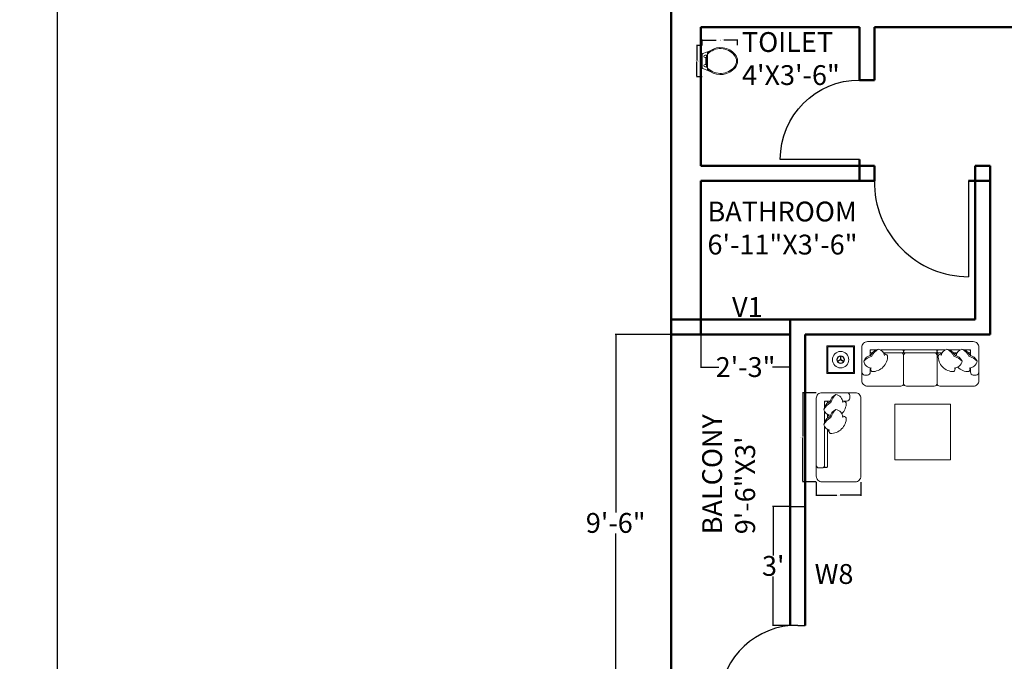
# Model space of a CAD drawing. Units: inches. Extents: x -173 to 545, y -746 to 104.
# Tile 21 of 32: x -173 to 125, y -321 to -127. Entities that reach past the tile are written whole.
import ezdxf

# ---------------------------------------------------------------- set-up
doc = ezdxf.new("R2010")
doc.units = ezdxf.units.IN
doc.header["$MEASUREMENT"] = 0
for name, color, linetype, lineweight in [('A-ANNO-DIMS', 2, 'Continuous', 18), ('A-ANNO-TEXT', 7, 'Continuous', 18), ('A-AREA-IDEN', 7, 'Continuous', 18), ('A-DOOR', 4, 'Continuous', 25), ('A-FLOR-FIXT', 8, 'Continuous', 18), ('A-FURN', 8, 'Continuous', 18), ('A-GLAZ', 3, 'Continuous', 25), ('A-WALL', 7, 'Continuous', 50)]:
    doc.layers.add(name, color=color, linetype=linetype, lineweight=lineweight)
doc.styles.get("Standard").update_dxf_attribs({"font": 'arial.ttf'})
doc.dimstyles.get("Standard").update_dxf_attribs({"dimtxt": 0.18, "dimasz": 0.18, "dimexe": 0.18, "dimexo": 0.0625, "dimgap": 0.09, "dimtad": 0, "dimtih": 1, "dimtoh": 1, "dimdec": 0, "dimzin": 0, "dimdsep": 46, "dimlunit": 3, "dimtxsty": 'Standard', "dimcen": 0.09, "dimadec": 0, "dimazin": 0, "dimtfac": 1, "dimtdec": 0, "dimtofl": 0, "dimtmove": 0, "dimatfit": 3, "dimfxl": 1, "dimtolj": 1, "dimtzin": 0, "dimarcsym": 0})

# ---------------------------------------------------------------- blocks, each defined once
blk = doc.blocks.new('*D2')
at = {"layer": 'A-ANNO-DIMS', "color": 0, "lineweight": -2, "transparency": 16777216}
for p, q in [((60.24, -273.86), (54.99, -273.86)), ((55.17, -274.04), (55.17, -288.71)), ((55.17, -309.68), (55.17, -295.02)), ((60.24, -309.86), (54.99, -309.86))]:
    blk.add_line(p, q, dxfattribs=at)
at = {"layer": 'A-ANNO-DIMS', "color": 0, "transparency": 16777216}
for points in [[(55.14, -274.04), (55.2, -274.04), (55.17, -273.86)], [(55.14, -309.68), (55.2, -309.68), (55.17, -309.86)]]:
    blk.add_solid(points, dxfattribs=at)
at = {"layer": 'Defpoints', "color": 0, "transparency": 16777216}
for p in [(60.3, -273.86), (55.17, -309.86), (60.3, -309.86)]:
    blk.add_point(p, dxfattribs=at)
at = {"layer": 'A-ANNO-DIMS', "color": 0, "transparency": 16777216, "insert": (55.17, -291.86), "char_height": 6, "attachment_point": 5}
blk.add_mtext("\\A1;3'", dxfattribs=at)
blk = doc.blocks.new('*D3')
at = {"layer": 'A-ANNO-DIMS', "color": 0, "lineweight": -2, "transparency": 16777216}
for p, q in [((33.3, -221.92), (33.3, -231.89)), ((60.3, -221.92), (60.3, -231.89)), ((33.48, -231.71), (38.69, -231.71)), ((60.12, -231.71), (54.92, -231.71))]:
    blk.add_line(p, q, dxfattribs=at)
at = {"layer": 'A-ANNO-DIMS', "color": 0, "transparency": 16777216}
for points in [[(33.48, -231.68), (33.48, -231.74), (33.3, -231.71)], [(60.12, -231.68), (60.12, -231.74), (60.3, -231.71)]]:
    blk.add_solid(points, dxfattribs=at)
at = {"layer": 'Defpoints', "color": 0, "transparency": 16777216}
for p in [(33.3, -221.86), (60.3, -221.86), (60.3, -231.71)]:
    blk.add_point(p, dxfattribs=at)
at = {"layer": 'A-ANNO-DIMS', "color": 0, "transparency": 16777216, "insert": (46.8, -231.71), "char_height": 6, "attachment_point": 5}
blk.add_mtext('\\A1;2\'-3"', dxfattribs=at)
blk = doc.blocks.new('*D7')
at = {"layer": 'A-ANNO-DIMS', "color": 0, "lineweight": -2, "transparency": 16777216}
for p, q in [((24.24, -221.86), (7.32, -221.86)), ((7.5, -222.04), (7.5, -275.71)), ((7.5, -335.68), (7.5, -282.02)), ((24.24, -335.86), (7.32, -335.86))]:
    blk.add_line(p, q, dxfattribs=at)
at = {"layer": 'A-ANNO-DIMS', "color": 0, "transparency": 16777216}
for points in [[(7.47, -222.04), (7.53, -222.04), (7.5, -221.86)], [(7.47, -335.68), (7.53, -335.68), (7.5, -335.86)]]:
    blk.add_solid(points, dxfattribs=at)
at = {"layer": 'Defpoints', "color": 0, "transparency": 16777216}
for p in [(24.3, -221.86), (7.5, -335.86), (24.3, -335.86)]:
    blk.add_point(p, dxfattribs=at)
at = {"layer": 'A-ANNO-DIMS', "color": 0, "transparency": 16777216, "insert": (7.5, -278.86), "char_height": 6, "attachment_point": 5}
blk.add_mtext('\\A1;9\'-6"', dxfattribs=at)
blk = doc.blocks.new('DAY BED1')
at = {"color": 0}
blk.add_line((0.3, 0.25), (0.225, 0.255), dxfattribs=at)
blk.add_lwpolyline([(-0.3, 0, -0.414214), (-0.4, 0.1), (-0.4, 0.1, 0.317837), (-0.4, 0.1, -0.414214), (-0.4, 0.1), (-0.4, 0.1, 1.186185), (-0.4, 0.1, -0.414214), (-0.4, 0.1), (-0.4, 1.5, -0.414214), (-0.3, 1.6), (0.3, 1.6, -0.414214), (0.4, 1.5), (0.4, 0.1, -0.414214), (0.3, 0)], format="xyb", close=True, dxfattribs=at)
for points in [[(-0.073, 1.45), (-0.15, 1.45, -0.414214), (-0.2, 1.5), (-0.2, 1.55, -0.414214), (-0.15, 1.6)], [(-0.073, 1.45, 0.165541), (-0.139, 1.419, 0.200231), (-0.058, 1.221, 0.121523)], [(-0.076, 1.425, -0.356772), (0.05, 1.568, -0.249542), (0.154, 1.438, 9.61688)], [(0.05, 1.568, -0.14773), (0.136, 1.422, -0.213343), (0.262, 1.293, -0.178662)], [(0.143, 1.442, -0.306663), (0.262, 1.293, -0.30633), (0.154, 1.196, 0.872847)], [(0.25, 1.345), (0.25, 1.45), (0.152, 1.45, -0.414214)], [(0.2, 1.412), (0.2, 1.43, -0.414214), (0.22, 1.45), (0.23, 1.45, -0.414214), (0.25, 1.43)], [(0.25, 1.43), (0.25, 1.345, -0.414214)], [(-0.076, 1.156, -0.356772), (0.05, 1.299, -0.249542), (0.154, 1.169, 9.61688)], [(0.05, 1.299, -0.14773), (0.136, 1.153, -0.213343), (0.262, 1.024, -0.178662)], [(0.25, 1.262), (0.25, 1.075, -0.414214)], [(-0.073, 1.181, 0.165541), (-0.139, 1.15, 0.425989), (0.148, 0.869, 0.121523), (0.187, 0.936, -7.115464)], [(0.143, 1.173, -0.306663), (0.262, 1.024, -0.30633), (0.154, 0.926, 0.872847)], [(0.168, 1.163, 0.071865), (0.187, 1.205, -7.115464)], [(0.2, 1.142), (0.2, 1.211, -0.414214)], [(0.25, 0.992), (0.25, 0.275, -0.414214), (0.23, 0.255), (0.22, 0.255, -0.414214), (0.2, 0.275), (0.2, 0.942, -0.414214)], [(0.25, 0.377), (0.25, 0.3, 0.414214), (0.3, 0.25), (0.35, 0.25, 0.414214), (0.4, 0.3)]]:
    blk.add_lwpolyline(points, format="xyb", dxfattribs=at)
for points in [[(0.25, 1.075), (0.25, 1.262)], [(0.25, 0.377), (0.25, 0.992)]]:
    blk.add_lwpolyline(points, dxfattribs=at)
blk = doc.blocks.new('*D24')
at = {"layer": 'A-ANNO-DIMS', "color": 0, "lineweight": -2, "transparency": 16777216}
for p, q in [((24.24, 16.64), (-161.72, 16.64)), ((-161.54, 16.46), (-161.54, -337.21)), ((-161.54, -697.18), (-161.54, -343.52)), ((24.24, -697.36), (-161.72, -697.36))]:
    blk.add_line(p, q, dxfattribs=at)
at = {"layer": 'A-ANNO-DIMS', "color": 0, "transparency": 16777216}
for points in [[(-161.57, 16.46), (-161.51, 16.46), (-161.54, 16.64)], [(-161.57, -697.18), (-161.51, -697.18), (-161.54, -697.36)]]:
    blk.add_solid(points, dxfattribs=at)
at = {"layer": 'Defpoints', "color": 0, "transparency": 16777216}
for p in [(24.3, 16.64), (-161.54, -697.36), (24.3, -697.36)]:
    blk.add_point(p, dxfattribs=at)
at = {"layer": 'A-ANNO-DIMS', "color": 0, "transparency": 16777216, "insert": (-161.54, -340.36), "char_height": 6, "attachment_point": 5}
blk.add_mtext('\\A1;59\'-6"', dxfattribs=at)
blk = doc.blocks.new('WC-COMPACT')
for p, q in [((1.62, 6.19), (1.62, 6.64)), ((1.62, 6.19), (1.62, 4.09)), ((1.62, 1.98), (1.62, 4.09)), ((1.62, 1.53), (1.62, 1.98))]:
    blk.add_line(p, q)
for points in [[(0, 4.09), (0, 6.13, -0.31031), (0.17, 6.38), (2.36, 7.22, -0.209071)], [(1.3, 5.82, -0.022712), (1.62, 6.19, -0.162618)], [(1.62, 6.19, -0.448546), (9.69, 5.9, -0.162618), (10.38, 4.09, -0.470877)], [(1.62, 6.64, -0.040937), (2.36, 7.22, -0.163732)], [(2.36, 7.22, -0.383919), (9.93, 6.1, -0.163732), (10.7, 4.09, -0.359733)], [(0, 4.09), (0, 2.04, 0.31031), (0.17, 1.79), (2.36, 0.95, 0.209071)], [(1.3, 5.82), (0.85, 5.82, 1), (0.85, 5.14), (1.08, 5.14)], [(1.3, 2.35), (0.85, 2.35, -1), (0.85, 3.03), (1.08, 3.03)], [(1.3, 4.09), (1.3, 5.82, -0.476108)], [(1.3, 4.09), (1.3, 2.35, 0.022712)], [(1.84, 1.77, 0.431639), (9.69, 2.28, 0.162618), (10.38, 4.09, 0.470877)], [(2.36, 0.95, 0.383919), (9.93, 2.08, 0.163732), (10.7, 4.09, 0.359733)], [(1.3, 2.35, 0.022712), (1.62, 1.98, 0.162618)], [(1.62, 1.98, 0.014165), (1.84, 1.77, 0.162618)], [(1.62, 1.53, 0.040937), (2.36, 0.95, 0.163732)]]:
    blk.add_lwpolyline(points, format="xyb")
for points in [[(1.08, 5.14), (1.08, 3.03)], [(1.08, 5.14), (1.3, 5.14)], [(1.08, 3.03), (1.3, 3.03)]]:
    blk.add_lwpolyline(points)
blk = doc.blocks.new('DOOR-24')
blk.add_line((24, 0), (24, 24))
blk.add_arc((24, 0), 24, 90, 180)
blk = doc.blocks.new('DOOR-BATH-29')
for p, q in [((28.5, 29), (28.5, 5)), ((28.5, 5), (28.5, 0))]:
    blk.add_line(p, q)
blk.add_arc((28.5, 28.5), 28.5, 179.0036, 270)
blk = doc.blocks.new('*D44')
at = {"layer": 'A-ANNO-DIMS', "color": 0, "lineweight": -2, "transparency": 16777216}
for p, q in [((68.14, -239.46), (63.98, -239.46)), ((64.16, -239.64), (64.16, -252.76)), ((64.16, -266.24), (64.16, -253.12)), ((68.14, -266.42), (63.98, -266.42))]:
    blk.add_line(p, q, dxfattribs=at)
at = {"layer": 'A-ANNO-DIMS', "color": 0, "transparency": 16777216}
for points in [[(64.13, -239.64), (64.19, -239.64), (64.16, -239.46)], [(64.13, -266.24), (64.19, -266.24), (64.16, -266.42)]]:
    blk.add_solid(points, dxfattribs=at)
at = {"layer": 'Defpoints', "color": 0, "transparency": 16777216}
for p in [(64.16, -239.46), (68.2, -239.46), (68.2, -266.42)]:
    blk.add_point(p, dxfattribs=at)
at = {"layer": 'A-ANNO-DIMS', "color": 0, "transparency": 16777216, "insert": (64.16, -252.94), "char_height": 0.18, "attachment_point": 5}
blk.add_mtext('\\A1;DAY BED 2\'-3"', dxfattribs=at)
blk = doc.blocks.new('*D45')
at = {"layer": 'A-ANNO-DIMS', "color": 0, "lineweight": -2, "transparency": 16777216}
for p, q in [((68.2, -266.49), (68.2, -270.65)), ((81.68, -266.49), (81.68, -270.65)), ((68.38, -270.47), (74.41, -270.47)), ((81.5, -270.47), (75.47, -270.47))]:
    blk.add_line(p, q, dxfattribs=at)
at = {"layer": 'A-ANNO-DIMS', "color": 0, "transparency": 16777216}
for points in [[(68.38, -270.44), (68.38, -270.5), (68.2, -270.47)], [(81.5, -270.44), (81.5, -270.5), (81.68, -270.47)]]:
    blk.add_solid(points, dxfattribs=at)
at = {"layer": 'Defpoints', "color": 0, "transparency": 16777216}
for p in [(68.2, -266.42), (81.68, -266.42), (68.2, -270.47)]:
    blk.add_point(p, dxfattribs=at)
at = {"layer": 'A-ANNO-DIMS', "color": 0, "transparency": 16777216, "insert": (74.94, -270.47), "char_height": 0.18, "attachment_point": 5}
blk.add_mtext('\\A1;1\'-1 1/2"', dxfattribs=at)
blk = doc.blocks.new('*D64')
at = {"layer": 'A-ANNO-DIMS', "color": 0, "lineweight": -2, "transparency": 16777216}
for p, q in [((33.69, -134.3), (33.69, -132.58)), ((33.87, -132.76), (37.88, -132.76)), ((44.22, -132.76), (40.21, -132.76)), ((44.4, -134.3), (44.4, -132.58))]:
    blk.add_line(p, q, dxfattribs=at)
at = {"layer": 'A-ANNO-DIMS', "color": 0, "transparency": 16777216}
for points in [[(33.87, -132.73), (33.87, -132.79), (33.69, -132.76)], [(44.22, -132.73), (44.22, -132.79), (44.4, -132.76)]]:
    blk.add_solid(points, dxfattribs=at)
at = {"layer": 'Defpoints', "color": 0, "transparency": 16777216}
for p in [(44.4, -132.76), (33.69, -134.37), (44.4, -134.37)]:
    blk.add_point(p, dxfattribs=at)
at = {"layer": 'A-ANNO-DIMS', "color": 0, "transparency": 16777216, "insert": (39.04, -132.76), "char_height": 0.18, "attachment_point": 5}
blk.add_mtext('\\A1;WC 0\'-10 1/2" TYP.', dxfattribs=at)
blk = doc.blocks.new('*D65')
at = {"layer": 'A-ANNO-DIMS', "color": 0, "lineweight": -2, "transparency": 16777216}
for p, q in [((33.63, -134.37), (31.91, -134.37)), ((32.09, -134.55), (32.09, -138.94)), ((32.09, -143.7), (32.09, -139.3)), ((33.63, -143.88), (31.91, -143.88))]:
    blk.add_line(p, q, dxfattribs=at)
at = {"layer": 'A-ANNO-DIMS', "color": 0, "transparency": 16777216}
for points in [[(32.06, -134.55), (32.12, -134.55), (32.09, -134.37)], [(32.06, -143.7), (32.12, -143.7), (32.09, -143.88)]]:
    blk.add_solid(points, dxfattribs=at)
at = {"layer": 'Defpoints', "color": 0, "transparency": 16777216}
for p in [(32.09, -134.37), (33.69, -134.37), (33.69, -143.88)]:
    blk.add_point(p, dxfattribs=at)
at = {"layer": 'A-ANNO-DIMS', "color": 0, "transparency": 16777216, "insert": (32.09, -139.12), "char_height": 0.18, "attachment_point": 5}
blk.add_mtext('\\A1;0\'-9 1/2" TYP.', dxfattribs=at)

msp = doc.modelspace()

# ---------------------------------------------------------------- linework, layer by layer
at = {"layer": 'A-DOOR'}
msp.add_arc((62.77, -333.86), 24.13, 95.876, 180, dxfattribs=at)
at = {"layer": 'A-FURN'}
for p, q in [((75.55, -229.42), (74.52, -230.01)), ((75.52, -229.47), (75.52, -228.28)), ((75.6, -229.42), (76.63, -230.01)), ((75.63, -229.47), (75.63, -228.28)), ((75.6, -229.51), (74.57, -230.11)), ((75.55, -229.51), (76.58, -230.11))]:
    msp.add_line(p, q, dxfattribs=at)
at = {"layer": 'A-FURN', "ltscale": 0.03}
for points in [[(71.36, -233.68), (79.79, -233.68), (79.79, -225.25), (71.36, -225.25)], [(108.85, -259.8), (92, -259.8), (92, -242.95), (108.85, -242.95)]]:
    msp.add_lwpolyline(points, close=True, dxfattribs=at)
at = {"layer": 'A-FURN'}
msp.add_lwpolyline([(79.45, -233.34), (71.7, -233.34), (71.7, -225.59), (79.45, -225.59)], close=True, dxfattribs=at)
at = {"layer": 'A-FURN', "ltscale": 0.03}
msp.add_lwpolyline([(82, -235.81, 0.414214), (83.69, -237.49), (93.8, -237.49, 0.414214), (94.64, -236.65, 0.414214), (95.48, -237.49), (103.91, -237.49, 0.414214), (104.75, -236.65, 0.414214), (105.59, -237.49), (115.7, -237.49, 0.414214), (117.39, -235.81), (117.39, -225.7, 0.414214), (115.7, -224.01), (83.69, -224.01, 0.414214), (82, -225.7)], format="xyb", close=True, dxfattribs=at)
at = {"layer": 'A-FURN'}
for points in [[(82.54, -229.9, -0.14773), (85, -228.45, -0.213343), (87.17, -226.33, -0.178662)], [(84.66, -228.34, -0.306663), (87.17, -226.33, -0.30633), (88.81, -228.16, 0.872847)], [(110.19, -228.34, 0.306663), (107.68, -226.33, 0.30633), (106.03, -228.16, -0.872847)], [(112.31, -229.9, 0.14773), (109.85, -228.45, 0.213343), (107.68, -226.33, 0.178662)], [(114.73, -228.34, 0.306663), (112.21, -226.33, 0.30633), (110.57, -228.16, -0.872847)], [(116.85, -229.9, 0.14773), (114.39, -228.45, 0.213343), (112.21, -226.33, 0.178662)], [(84.95, -232.03, -0.356772), (82.54, -229.9, -0.249542), (84.72, -228.15, 9.61688)], [(85.17, -227.38), (84.87, -227.38, -0.414214), (84.53, -227.05), (84.53, -226.88, -0.414214), (84.87, -226.54)], [(84.53, -231.97, 0.165541), (85.05, -233.09, 0.425989), (89.78, -228.26, 0.121523), (88.66, -227.6, -7.115464)], [(84.87, -226.54), (86.3, -226.54, -0.414214)], [(87.7, -226.54), (94.3, -226.54, -0.414214), (94.64, -226.88), (94.64, -227.05, -0.414214), (94.3, -227.38), (88.55, -227.38, -0.414214)], [(93.8, -227.38, -0.414214), (94.64, -228.23), (94.64, -236.65, -0.414214)], [(95.48, -227.38, 0.414214), (94.64, -228.23)], [(103.91, -227.38, -0.414214), (104.75, -228.23)], [(107.15, -226.54), (105.09, -226.54, 0.414214), (104.75, -226.88), (104.75, -227.05, 0.414214), (105.09, -227.38), (106.3, -227.38, 0.414214)], [(105.59, -227.38, 0.414214), (104.75, -228.23), (104.75, -236.65, 0.414214)], [(110.32, -231.97, -0.165541), (109.8, -233.09, -0.425989), (105.07, -228.26, -0.121523), (106.19, -227.6, 7.115464)], [(111.68, -226.54), (108.55, -226.54, 0.414214)], [(109.68, -227.38), (110.84, -227.38, 0.414214)], [(109.9, -232.03, 0.356772), (112.31, -229.9, 0.249542), (110.12, -228.15, -9.61688)], [(110.02, -227.93, -0.071865), (110.73, -227.6, 7.115464)], [(113.09, -226.54), (114.86, -226.54), (114.86, -228.2, 0.414214)], [(114.52, -226.54), (113.09, -226.54, 0.414214)], [(114.22, -227.38), (114.52, -227.38, 0.414214), (114.86, -227.05), (114.86, -226.88, 0.414214), (114.52, -226.54)], [(114.44, -232.03, 0.356772), (116.85, -229.9, 0.249542), (114.66, -228.15, -9.61688)], [(82, -233.28, 0.414214), (82.84, -234.12), (83.69, -234.12, 0.414214), (84.53, -233.28), (84.53, -231.97)], [(114.86, -231.97, -0.165541), (114.34, -233.09, -0.200231), (110.99, -231.73, -0.121523)], [(114.86, -231.97), (114.86, -233.28, 0.414214), (115.7, -234.12), (116.54, -234.12, 0.414214), (117.39, -233.28)]]:
    msp.add_lwpolyline(points, format="xyb", dxfattribs=at)
for points in [[(84.53, -228.2), (84.53, -226.54), (86.3, -226.54)], [(87.7, -226.54), (107.15, -226.54)], [(108.55, -226.54), (111.68, -226.54)]]:
    msp.add_lwpolyline(points, dxfattribs=at)
msp.add_lwpolyline([(104.41, -226.54), (94.98, -226.54, 0.414214), (94.64, -226.88), (94.64, -227.05, 0.414214), (94.98, -227.38), (104.41, -227.38, 0.414214), (104.75, -227.05), (104.75, -226.88, 0.414214)], format="xyb", close=True, dxfattribs=at)
for radius in [2.48, 1.19, 1.07]:
    msp.add_circle((75.57, -229.47), radius, dxfattribs=at)
at = {"layer": 'A-GLAZ'}
for p, q in [((60.3, -273.86), (64.8, -273.86)), ((62.64, -309.86), (60.3, -309.86)), ((62.64, -309.86), (64.8, -309.86))]:
    msp.add_line(p, q, dxfattribs=at)
at = {"layer": 'A-WALL'}
for p, q in [((24.3, 16.64), (24.3, -697.36)), ((33.3, -128.86), (81.3, -128.86)), ((33.3, -128.86), (33.3, -170.86)), ((81.3, -128.86), (81.3, -144.86)), ((85.8, -128.86), (85.8, -144.86)), ((85.8, -128.86), (139.3, -128.86)), ((81.3, -144.86), (85.8, -144.86)), ((81.3, -168.86), (81.3, -175.36)), ((33.3, -170.86), (85.8, -170.86)), ((85.8, -170.86), (85.8, -175.36)), ((116.3, -170.86), (116.3, -217.36)), ((116.3, -170.86), (120.8, -170.86)), ((120.8, -170.86), (120.8, -221.86)), ((33.3, -175.36), (85.8, -175.36)), ((33.3, -175.36), (33.3, -221.86)), ((114.3, -175.36), (120.8, -175.36)), ((24.3, -217.36), (116.3, -217.36)), ((60.3, -217.36), (60.3, -309.86)), ((24.3, -221.86), (60.3, -221.86)), ((64.8, -221.86), (64.8, -309.86)), ((64.8, -221.86), (69.3, -221.86)), ((69.3, -221.86), (69.3, -221.86)), ((69.3, -221.86), (73.8, -221.86)), ((73.8, -221.86), (120.8, -221.86))]:
    msp.add_line(p, q, dxfattribs=at)

# ---------------------------------------------------------------- block references
at = {"layer": 'A-DOOR', "extrusion": (0, 0, -1), "zscale": -1, "rotation": 270.0000000000001}
msp.add_blockref('DOOR-24', (-81.3, -144.86), dxfattribs=at)
at = {"layer": 'A-DOOR'}
msp.add_blockref('DOOR-BATH-29', (85.8, -204.36), dxfattribs=at)
at = {"layer": 'A-FLOR-FIXT'}
msp.add_blockref('WC-COMPACT', (33.69, -143.21), dxfattribs=at)
at = {"layer": 'A-FURN', "ltscale": 0.03, "xscale": -16.8499431786091, "yscale": 16.8499431786091, "zscale": 16.8499431786091}
msp.add_blockref('DAY BED1', (74.94, -266.42), dxfattribs=at)

# ---------------------------------------------------------------- texts
at = {"layer": 'A-ANNO-TEXT', "char_height": 6, "attachment_point": 1}
for s, insert in [('V1', (42.71, -210.54)), ('W8', (67.71, -291.31))]:
    msp.add_mtext(s, dxfattribs=dict(at, insert=insert))
at = {"layer": 'A-AREA-IDEN', "char_height": 6, "attachment_point": 1}
for s, insert in [('TOILET\\P4\'X3\'-6"', (45.72, -130.37)), ('BATHROOM\\P6\'-11"X3\'-6"', (35.28, -181.65))]:
    msp.add_mtext(s, dxfattribs=dict(at, insert=insert))
at = {"layer": 'A-AREA-IDEN', "insert": (33.68, -282.29), "char_height": 6, "attachment_point": 1, "rotation": 90}
msp.add_mtext('BALCONY\\P9\'-6"X3\'', dxfattribs=at)

# ---------------------------------------------------------------- dimensions: what is measured, and where the dimension line sits
at = {"layer": 'A-ANNO-DIMS'}
for base, p1, p2, angle, override, picture, middle in [((-161.54, -697.36), (24.3, 16.64), (24.3, -697.36), 90, {"dimtxt": 6, "dimclrd": 0, "dimclre": 0, "dimclrt": 0}, '*D24', (-161.54, -340.36)), ((7.5, -335.86), (24.3, -221.86), (24.3, -335.86), 90, {"dimtxt": 6, "dimclrd": 0, "dimclre": 0, "dimclrt": 0}, '*D7', (7.5, -278.86)), ((68.2, -270.47), (81.68, -266.42), (68.2, -266.42), 180, {"dimdec": 1, "dimlfac": 1, "dimrnd": 0, "dimzin": 1, "dimdsep": 46, "dimlunit": 4, "dimfrac": 2}, '*D45', (74.94, -270.47)), ((55.17, -309.86), (60.3, -273.86), (60.3, -309.86), 90, {"dimtxt": 6, "dimclrd": 0, "dimclre": 0, "dimclrt": 0}, '*D2', (55.17, -291.86))]:
    dim = msp.add_linear_dim(base=base, p1=p1, p2=p2, angle=angle, dimstyle='Standard', override=override, dxfattribs=at)
    dim.commit()
    dim.dimension.update_dxf_attribs({"geometry": picture, "text_midpoint": middle})
dim = msp.add_linear_dim(base=(44.4, -132.76), p1=(33.69, -134.37), p2=(44.4, -134.37), text='WC <> TYP.', dimstyle='Standard', override={"dimdec": 1, "dimlfac": 1, "dimrnd": 0, "dimzin": 1, "dimdsep": 46, "dimlunit": 4, "dimfrac": 2}, dxfattribs=at)
dim.commit()
dim.dimension.update_dxf_attribs({"geometry": '*D64', "text_midpoint": (39.04, -132.76)})
for base, p1, p2, text, picture, middle in [((32.09, -134.37), (33.69, -143.88), (33.69, -134.37), '<> TYP.', '*D65', (32.09, -139.12)), ((64.16, -239.46), (68.2, -266.42), (68.2, -239.46), 'DAY BED <>', '*D44', (64.16, -252.94))]:
    dim = msp.add_linear_dim(base=base, p1=p1, p2=p2, angle=90, text=text, dimstyle='Standard', override={"dimdec": 1, "dimlfac": 1, "dimrnd": 0, "dimzin": 1, "dimdsep": 46, "dimlunit": 4, "dimfrac": 2}, dxfattribs=at)
    dim.commit()
    dim.dimension.update_dxf_attribs({"geometry": picture, "text_midpoint": middle})
dim = msp.add_linear_dim(base=(60.3, -231.71), p1=(33.3, -221.86), p2=(60.3, -221.86), dimstyle='Standard', override={"dimtxt": 6, "dimclrd": 0, "dimclre": 0, "dimclrt": 0}, dxfattribs=at)
dim.commit()
dim.dimension.update_dxf_attribs({"geometry": '*D3', "text_midpoint": (46.8, -231.71)})

doc.saveas('drawing.dxf')
